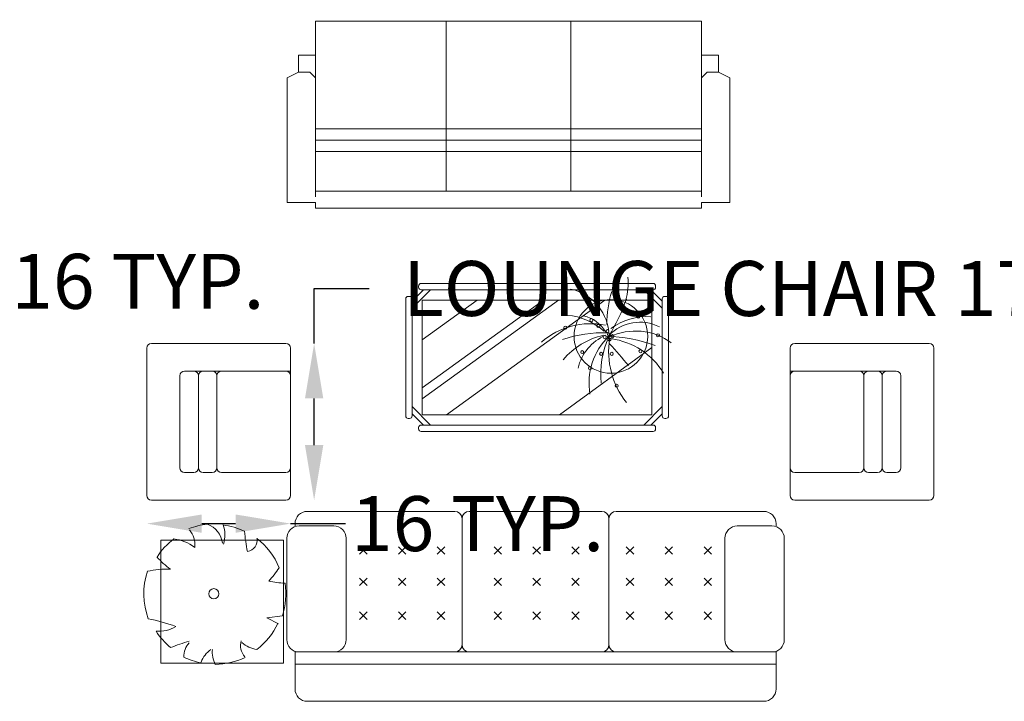
# Model space of a CAD drawing. Units: inches. Extents: x 1994 to 3075, y 3517 to 3950.
# Tile 55 of 58: x 2912 to 3019, y 3623 to 3698. Entities that reach past the tile are written whole.
import ezdxf

# ---------------------------------------------------------------- set-up
doc = ezdxf.new("R2010")
doc.units = ezdxf.units.IN
doc.layers.add('A-ANNO-DIMS', color=2, linetype='Continuous', lineweight=18)
doc.layers.add('A-FURN', color=8, linetype='Continuous', lineweight=18)
doc.styles.get("Standard").update_dxf_attribs({"font": 'arial.ttf'})
doc.dimstyles.get("Standard").update_dxf_attribs({"dimtxt": 6, "dimasz": 6, "dimexe": 0.18, "dimexo": 0.0625, "dimgap": 0.09, "dimtad": 0, "dimtih": 1, "dimtoh": 1, "dimdec": 4, "dimzin": 0, "dimdsep": 46, "dimlunit": 4, "dimtxsty": 'Standard', "dimcen": 0.09, "dimse1": 1, "dimse2": 1, "dimadec": 0, "dimazin": 0, "dimtfac": 1, "dimtdec": 4, "dimtofl": 0, "dimtmove": 0, "dimatfit": 3, "dimfxl": 1, "dimtolj": 1, "dimtzin": 0, "dimarcsym": 0})

# ---------------------------------------------------------------- blocks, each defined once
blk = doc.blocks.new('CHAIR-LOUNGE')
for p, q in [((0, 16.6), (0, 0.5)), ((0.5, 17.1), (15.19, 17.1)), ((15.7, 16.6), (15.7, 0.5)), ((4.12, 14.09), (15.7, 14.09)), ((3.62, 13.58), (3.62, 3.52)), ((5.63, 13.58), (5.63, 3.52)), ((7.65, 3.52), (7.65, 13.58)), ((4.12, 3.02), (5.13, 3.02)), ((6.14, 3.02), (7.14, 3.02)), ((8.15, 3.02), (15.19, 3.02)), ((0.5, 0), (15.19, 0))]:
    blk.add_line(p, q)
for centre, start, end in [((0.5, 16.6), 90, 180), ((15.19, 16.6), 0, 90), ((4.12, 13.58), 90, 180), ((5.13, 13.58), 0, 90), ((6.14, 13.58), 90, 180), ((7.14, 13.58), 0, 90), ((8.15, 13.58), 90, 180), ((15.19, 13.58), 0, 90), ((4.12, 3.52), 180, 270), ((5.13, 3.52), 270, 0), ((6.14, 3.52), 180, 270), ((7.14, 3.52), 270, 0), ((8.15, 3.52), 180, 270), ((15.19, 3.52), 270, 0), ((0.5, 0.5), 180, 270), ((15.19, 0.5), 270, 0)]:
    blk.add_arc(centre, 0.503, start, end)
blk = doc.blocks.new('*D15')
at = {"layer": 'A-ANNO-DIMS', "color": 0, "lineweight": -2, "transparency": 16777216}
for p, q in [((2835.85, 3669.06), (2840.19, 3669.06)), ((2846.19, 3669.06), (2852.19, 3669.06))]:
    blk.add_line(p, q, dxfattribs=at)
at = {"layer": 'A-ANNO-DIMS', "color": 0, "transparency": 16777216}
for points in [[(2835.85, 3670.06), (2835.85, 3668.06), (2829.85, 3669.06)], [(2840.19, 3670.06), (2840.19, 3668.06), (2846.19, 3669.06)]]:
    blk.add_solid(points, dxfattribs=at)
at = {"layer": 'Defpoints', "color": 0, "transparency": 16777216}
for p in [(2829.85, 3671.51), (2846.19, 3671.51), (2846.19, 3669.06)]:
    blk.add_point(p, dxfattribs=at)
at = {"layer": 'A-ANNO-DIMS', "color": 0, "transparency": 16777216, "insert": (2896.77, 3669.06), "char_height": 6, "attachment_point": 5}
blk.add_mtext('\\A1;DINING CHAIR 16 TYP.', dxfattribs=at)
blk = doc.blocks.new('*D25')
at = {"layer": 'A-ANNO-DIMS', "color": 0, "lineweight": -2, "transparency": 16777216}
for p, q in [((2943.67, 3662.28), (2943.67, 3668.28)), ((2943.67, 3668.28), (2949.67, 3668.28)), ((2943.67, 3651.18), (2943.67, 3656.28))]:
    blk.add_line(p, q, dxfattribs=at)
at = {"layer": 'A-ANNO-DIMS', "color": 0, "transparency": 16777216}
for points in [[(2942.67, 3656.28), (2944.67, 3656.28), (2943.67, 3662.28)], [(2942.67, 3651.18), (2944.67, 3651.18), (2943.67, 3645.18)]]:
    blk.add_solid(points, dxfattribs=at)
at = {"layer": 'Defpoints', "color": 0, "transparency": 16777216}
for p in [(2941.1, 3662.28), (2943.67, 3662.28), (2941.1, 3645.18)]:
    blk.add_point(p, dxfattribs=at)
at = {"layer": 'A-ANNO-DIMS', "color": 0, "transparency": 16777216, "insert": (2997.3, 3668.28), "char_height": 6, "attachment_point": 5}
blk.add_mtext('\\A1;LOUNGE CHAIR 17 TYP.', dxfattribs=at)
blk = doc.blocks.new('*D26')
at = {"layer": 'A-ANNO-DIMS', "color": 0, "lineweight": -2, "transparency": 16777216}
for p, q in [((2931.41, 3642.61), (2935.1, 3642.61)), ((2941.1, 3642.61), (2947.1, 3642.61))]:
    blk.add_line(p, q, dxfattribs=at)
at = {"layer": 'A-ANNO-DIMS', "color": 0, "transparency": 16777216}
for points in [[(2931.41, 3643.61), (2931.41, 3641.61), (2925.41, 3642.61)], [(2935.1, 3643.61), (2935.1, 3641.61), (2941.1, 3642.61)]]:
    blk.add_solid(points, dxfattribs=at)
at = {"layer": 'Defpoints', "color": 0, "transparency": 16777216}
for p in [(2925.41, 3645.18), (2941.1, 3645.18), (2941.1, 3642.61)]:
    blk.add_point(p, dxfattribs=at)
at = {"layer": 'A-ANNO-DIMS', "color": 0, "transparency": 16777216, "insert": (2961.51, 3642.61), "char_height": 6, "attachment_point": 5}
blk.add_mtext('\\A1;16 TYP.', dxfattribs=at)
blk = doc.blocks.new('*D27')
at = {"layer": 'A-ANNO-DIMS', "color": 0, "lineweight": -2, "transparency": 16777216}
for p, q in [((2981.58, 3712.96), (2981.58, 3712.87)), ((2981.58, 3706.38), (2981.58, 3706.48))]:
    blk.add_line(p, q, dxfattribs=at)
at = {"layer": 'A-ANNO-DIMS', "color": 0, "transparency": 16777216}
for points in [[(2980.58, 3712.96), (2982.58, 3712.96), (2981.58, 3718.96)], [(2980.58, 3706.38), (2982.58, 3706.38), (2981.58, 3700.38)]]:
    blk.add_solid(points, dxfattribs=at)
at = {"layer": 'Defpoints', "color": 0, "transparency": 16777216}
for p in [(2984.36, 3718.96), (2981.58, 3700.38), (2984.36, 3700.38)]:
    blk.add_point(p, dxfattribs=at)
at = {"layer": 'A-ANNO-DIMS', "color": 0, "transparency": 16777216, "insert": (2981.58, 3709.67), "char_height": 6, "attachment_point": 5}
blk.add_mtext('\\A1;SIDE CHAIR 19 TYP.', dxfattribs=at)

msp = doc.modelspace()

# ---------------------------------------------------------------- linework, layer by layer
at = {"layer": 'A-FURN'}
for p, q in [((2943.833, 3697.4715), (2943.833, 3678.2684)), ((2985.9559, 3697.4715), (2943.833, 3697.4715)), ((2958.0805, 3697.4715), (2958.0805, 3678.8879)), ((2971.7084, 3697.4715), (2971.7084, 3678.8879)), ((2985.9559, 3697.4715), (2985.9559, 3678.2684)), ((2943.833, 3693.7548), (2941.9746, 3693.7548)), ((2941.9746, 3693.7548), (2941.9746, 3691.8964)), ((2987.8143, 3693.7548), (2985.9559, 3693.7548)), ((2987.8143, 3691.8964), (2987.8143, 3693.7548)), ((2941.9746, 3691.8964), (2940.7357, 3691.277)), ((2941.9746, 3691.8964), (2943.2136, 3691.8964)), ((2943.2136, 3691.8964), (2943.833, 3691.277)), ((2986.5754, 3691.8964), (2985.9559, 3691.277)), ((2987.8143, 3691.8964), (2986.5754, 3691.8964)), ((2989.0532, 3691.277), (2987.8143, 3691.8964)), ((2940.7357, 3691.277), (2940.7357, 3677.649)), ((2989.0532, 3677.649), (2989.0532, 3691.277)), ((2985.9559, 3685.7019), (2943.833, 3685.7019)), ((2985.9559, 3684.463), (2943.833, 3684.463)), ((2985.9559, 3683.2241), (2943.833, 3683.2241)), ((2943.833, 3678.8879), (2985.9559, 3678.8879)), ((2940.7357, 3677.649), (2943.833, 3677.649)), ((2943.833, 3677.649), (2943.833, 3677.0295)), ((2943.833, 3677.0295), (2985.9559, 3677.0295)), ((2985.9559, 3677.0295), (2985.9559, 3677.649)), ((2985.9559, 3677.649), (2989.0532, 3677.649)), ((2956.3786, 3668.1312), (2954.3653, 3666.1179)), ((2955.5909, 3668.1312), (2954.3653, 3666.9056)), ((2955.0776, 3668.549), (2955.0776, 3668.4097)), ((2955.3561, 3668.8275), (2980.6682, 3668.8275)), ((2955.3561, 3668.1312), (2980.6682, 3668.1312)), ((2979.6457, 3668.1312), (2981.659, 3666.1179)), ((2980.4334, 3668.1312), (2981.659, 3666.9056)), ((2980.9467, 3668.549), (2980.9467, 3668.4097)), ((2953.669, 3654.3612), (2953.669, 3667.1404)), ((2953.9475, 3667.4189), (2954.0868, 3667.4189)), ((2954.3653, 3654.3612), (2954.3653, 3667.1404)), ((2981.659, 3667.1404), (2981.659, 3654.3612)), ((2982.0768, 3667.4189), (2981.9375, 3667.4189)), ((2982.3553, 3667.1404), (2982.3553, 3654.3612)), ((2955.4793, 3656.2225), (2970.3399, 3667.0172)), ((2955.4793, 3657.4188), (2968.693, 3667.0172)), ((2955.4793, 3662.6734), (2961.4592, 3667.0172)), ((2955.4793, 3654.4844), (2955.4793, 3667.0172)), ((2955.4793, 3667.0172), (2980.545, 3667.0172)), ((2958.1325, 3654.4844), (2975.3859, 3667.0172)), ((2980.545, 3667.0172), (2980.545, 3654.4844)), ((2970.4453, 3654.4844), (2980.545, 3661.8208)), ((2956.3786, 3653.3703), (2954.3653, 3655.3837)), ((2979.6457, 3653.3703), (2981.659, 3655.3837)), ((2955.5909, 3653.3703), (2954.3653, 3654.5959)), ((2980.545, 3654.4844), (2955.4793, 3654.4844)), ((2980.4334, 3653.3703), (2981.659, 3654.5959)), ((2953.9475, 3654.0827), (2954.0868, 3654.0827)), ((2955.0776, 3652.9526), (2955.0776, 3653.0918)), ((2980.6682, 3653.3703), (2955.3561, 3653.3703)), ((2980.9467, 3652.9526), (2980.9467, 3653.0918)), ((2982.0768, 3654.0827), (2981.9375, 3654.0827)), ((2980.6682, 3652.6741), (2955.3561, 3652.6741)), ((2942.932, 3643.9457), (2959.0378, 3643.9457)), ((2960.6024, 3643.9457), (2975.074, 3643.9457)), ((2976.6386, 3643.9457), (2992.7443, 3643.9457)), ((2941.5858, 3642.3608), (2941.5858, 3642.5995)), ((2942.0319, 3642.3608), (2945.8188, 3642.3608)), ((2959.8201, 3643.1384), (2959.8201, 3629.406)), ((2975.8563, 3643.1384), (2975.8563, 3629.406)), ((2993.6444, 3642.3608), (2989.8575, 3642.3608)), ((2994.0906, 3642.3608), (2994.0906, 3642.5995)), ((2926.9262, 3627.3737), (2926.9262, 3640.7908)), ((2926.9262, 3640.7908), (2940.3433, 3640.7908)), ((2940.3433, 3640.7908), (2940.3433, 3627.3737)), ((2940.6856, 3629.9445), (2940.6856, 3641.0145)), ((2947.1651, 3641.0145), (2947.1651, 3629.9445)), ((2988.5113, 3641.0145), (2988.5113, 3629.9445)), ((2994.9907, 3629.9445), (2994.9907, 3641.0145)), ((2949.4419, 3640.0866), (2948.6296, 3639.2743)), ((2948.6296, 3640.0866), (2949.4419, 3639.2743)), ((2953.6852, 3640.0866), (2952.8729, 3639.2743)), ((2952.8729, 3640.0866), (2953.6852, 3639.2743)), ((2957.9285, 3640.0866), (2957.1162, 3639.2743)), ((2957.1162, 3640.0866), (2957.9285, 3639.2743)), ((2963.309, 3640.0866), (2964.1213, 3639.2743)), ((2964.1213, 3640.0866), (2963.309, 3639.2743)), ((2967.5523, 3640.0866), (2968.3646, 3639.2743)), ((2968.3646, 3640.0866), (2967.5523, 3639.2743)), ((2971.7956, 3640.0866), (2972.6079, 3639.2743)), ((2972.6079, 3640.0866), (2971.7956, 3639.2743)), ((2978.5602, 3640.0866), (2977.7479, 3639.2743)), ((2977.7479, 3640.0866), (2978.5602, 3639.2743)), ((2982.8035, 3640.0866), (2981.9912, 3639.2743)), ((2981.9912, 3640.0866), (2982.8035, 3639.2743)), ((2987.0467, 3640.0866), (2986.2344, 3639.2743)), ((2986.2344, 3640.0866), (2987.0467, 3639.2743)), ((2949.4419, 3636.6669), (2948.6296, 3635.8546)), ((2948.6296, 3636.6669), (2949.4419, 3635.8546)), ((2953.6852, 3636.6669), (2952.8729, 3635.8546)), ((2952.8729, 3636.6669), (2953.6852, 3635.8546)), ((2957.9285, 3636.6669), (2957.1162, 3635.8546)), ((2957.1162, 3636.6669), (2957.9285, 3635.8546)), ((2963.309, 3636.6669), (2964.1213, 3635.8546)), ((2964.1213, 3636.6669), (2963.309, 3635.8546)), ((2967.5523, 3636.6669), (2968.3646, 3635.8546)), ((2968.3646, 3636.6669), (2967.5523, 3635.8546)), ((2971.7956, 3636.6669), (2972.6079, 3635.8546)), ((2972.6079, 3636.6669), (2971.7956, 3635.8546)), ((2978.5602, 3636.6669), (2977.7479, 3635.8546)), ((2977.7479, 3636.6669), (2978.5602, 3635.8546)), ((2982.8035, 3636.6669), (2981.9912, 3635.8546)), ((2981.9912, 3636.6669), (2982.8035, 3635.8546)), ((2987.0467, 3636.6669), (2986.2344, 3635.8546)), ((2986.2344, 3636.6669), (2987.0467, 3635.8546)), ((2949.4419, 3632.9736), (2948.6296, 3632.1613)), ((2948.6296, 3632.9736), (2949.4419, 3632.1613)), ((2952.8729, 3632.9736), (2953.6852, 3632.1613)), ((2953.6852, 3632.9736), (2952.8729, 3632.1613)), ((2957.9285, 3632.9736), (2957.1162, 3632.1613)), ((2957.1162, 3632.9736), (2957.9285, 3632.1613)), ((2963.309, 3632.9736), (2964.1213, 3632.1613)), ((2964.1213, 3632.9736), (2963.309, 3632.1613)), ((2968.3646, 3632.9736), (2967.5523, 3632.1613)), ((2967.5523, 3632.9736), (2968.3646, 3632.1613)), ((2971.7956, 3632.9736), (2972.6079, 3632.1613)), ((2972.6079, 3632.9736), (2971.7956, 3632.1613)), ((2978.5602, 3632.9736), (2977.7479, 3632.1613)), ((2977.7479, 3632.9736), (2978.5602, 3632.1613)), ((2981.9912, 3632.9736), (2982.8035, 3632.1613)), ((2982.8035, 3632.9736), (2981.9912, 3632.1613)), ((2987.0467, 3632.9736), (2986.2344, 3632.1613)), ((2986.2344, 3632.9736), (2987.0467, 3632.1613)), ((2940.2002, 3632.5581), (2938.4968, 3632.3296)), ((2938.4968, 3632.3296), (2939.7691, 3631.6814)), ((2941.5858, 3624.5594), (2941.5858, 3628.6743)), ((2994.0906, 3628.5982), (2941.5858, 3628.5982)), ((2994.0906, 3628.5982), (2994.0906, 3624.5594)), ((2940.3433, 3627.3737), (2926.9262, 3627.3737)), ((2994.0906, 3627.2519), (2941.5858, 3627.2519)), ((2992.7443, 3623.2131), (2942.932, 3623.2131))]:
    msp.add_line(p, q, dxfattribs=at)
for centre, radius in [((2976.0594, 3663.0507), 4.0196), ((2973.9283, 3664.8216), 0.1671), ((2979.0586, 3665.1899), 0.1671), ((2971.0956, 3663.9954), 0.1671), ((2974.6942, 3664.1795), 0.1671), ((2975.3826, 3662.985), 0.1671), ((2975.6895, 3663.6271), 0.1671), ((2975.843, 3663.2604), 0.1671), ((2975.919, 3662.7096), 0.1671), ((2976.2246, 3663.0763), 0.1671), ((2981.2014, 3663.1692), 0.1671), ((2972.9329, 3661.331), 0.1671), ((2974.9997, 3661.1469), 0.1671), ((2976.1485, 3661.1469), 0.1671), ((2979.2881, 3661.4223), 0.1671), ((2973.7748, 3659.5857), 0.1671), ((2976.6849, 3657.6563), 0.1671), ((2932.7283, 3634.9579), 0.5534)]:
    msp.add_circle(centre, radius, dxfattribs=at)
for centre, radius, start, end in [((2971.8422, 3668.819), 6.1066, 342.945635, 6.481378), ((2955.3561, 3668.549), 0.2785, 90, 180), ((2955.3561, 3668.4097), 0.2785, 180, 270), ((2970.5178, 3662.9741), 5.3651, 6.990448, 78.028363), ((2980.6682, 3668.549), 0.2785, 0, 90), ((2980.6682, 3668.4097), 0.2785, 270, 0), ((2953.9475, 3667.1404), 0.2785, 90, 180), ((2954.0868, 3667.1404), 0.2785, 0, 90), ((2989.2543, 3664.1518), 13.6438, 163.856122, 179.110515), ((2956.4997, 3674.7047), 22.5695, 328.987278, 340.361011), ((2981.9375, 3667.1404), 0.2785, 90, 180), ((2982.0768, 3667.1404), 0.2785, 0, 90), ((2970.5544, 3658.2067), 7.2086, 48.758099, 83.862401), ((2972.3832, 3661.838), 3.5142, 28.890119, 78.457922), ((2979.9704, 3658.7231), 6.4836, 85.874061, 126.95584), ((2973.8412, 3656.2772), 8.1559, 78.551551, 130.981535), ((2979.2198, 3659.898), 4.7015, 62.990858, 135.910172), ((2975.2814, 3649.4586), 13.9919, 88.328565, 108.729003), ((2977.0604, 3655.2659), 8.1127, 103.045235, 139.776625), ((2977.6244, 3658.3297), 5.3014, 114.095577, 166.295338), ((2980.9118, 3657.9156), 7.2337, 134.486062, 189.376218), ((2984.571, 3658.9315), 9.6234, 155.08876, 185.963724), ((2974.9332, 3645.2045), 17.8846, 70.524897, 87.824368), ((2984.8705, 3661.4231), 9.0569, 171.249582, 218.23328), ((2978.7571, 3657.1046), 6.5295, 53.32313, 115.763258), ((2974.9779, 3654.8745), 8.0016, 31.315049, 82.137794), ((2939.2692, 3628.4544), 49.8533, 39.04877, 42.6799), ((2953.9475, 3654.3612), 0.2785, 180, 270), ((2954.0868, 3654.3612), 0.2785, 270, 0), ((2981.9375, 3654.3612), 0.2785, 180, 270), ((2982.0768, 3654.3612), 0.2785, 270, 0), ((2955.3561, 3653.0918), 0.2785, 90, 180), ((2980.6682, 3653.0918), 0.2785, 0, 90), ((2955.3561, 3652.9526), 0.2785, 180, 270), ((2980.6682, 3652.9526), 0.2785, 270, 0), ((2942.932, 3642.5995), 1.3463, 90, 180), ((2959.0123, 3643.1384), 0.8078, 0, 90), ((2960.6278, 3643.1384), 0.8078, 90, 180), ((2975.0485, 3643.1384), 0.8078, 0, 90), ((2976.664, 3643.1384), 0.8078, 90, 180), ((2992.7443, 3642.5995), 1.3463, 0, 90), ((2932.8043, 3634.9551), 7.6406, 95.923625, 111.527702), ((2931.1212, 3640.1371), 2.578, 7.391154, 69.695169), ((2932.8043, 3634.9551), 7.5625, 64.349833, 83.035621), ((2930.7372, 3641.3713), 3.1922, 341.800851, 20.599149), ((2942.0319, 3641.0145), 1.3463, 90, 180), ((2945.8188, 3641.0145), 1.3463, 0, 90), ((2989.8575, 3641.0145), 1.3463, 90, 180), ((2993.6444, 3641.0145), 1.3463, 0, 90), ((2928.286, 3640.3558), 2.3685, 351.831375, 41.827816), ((2952.089, 3642.9331), 16.053, 184.146464, 192.123814), ((2932.8043, 3634.9551), 7.4492, 126.594039, 147.446376), ((2927.9323, 3636.608), 4.3493, 51.658233, 84.30928), ((2936.1976, 3640.81), 1.2638, 278.94104, 10.010745), ((2932.8043, 3634.9551), 7.5966, 22.010297, 52.639163), ((2932.4927, 3644.1371), 7.9007, 220.853588, 235.192991), ((2932.8043, 3634.9551), 7.7319, 161.530732, 200.629966), ((2927.6423, 3628.1563), 9.4998, 87.945495, 103.214626), ((2932.5958, 3642.2403), 8.5018, 315.978173, 328.531467), ((2941.236, 3648.8328), 12.7534, 258.572822, 266.664893), ((2932.8043, 3634.9551), 7.7746, 342.042609, 8.475005), ((2919.4257, 3604.4203), 28.4809, 71.286489, 77.545106), ((2932.8043, 3634.9551), 7.6324, 307.275083, 334.82454), ((2926.7274, 3634.2385), 3.3843, 264.732262, 302.854398), ((2932.8043, 3634.9551), 7.583, 212.609838, 230.67525), ((2936.8081, 3607.1269), 23.6509, 106.639749, 111.909938), ((2931.6696, 3628.0771), 2.227, 137.045394, 180.965052), ((2937.5176, 3629.3175), 1.8838, 164.855493, 220.959999), ((2937.8954, 3632.0995), 3.2517, 229.720325, 261.715134), ((2942.0319, 3629.9445), 1.3463, 180, 270), ((2945.8188, 3629.9445), 1.3463, 270, 0), ((2989.8575, 3629.9445), 1.3463, 180, 270), ((2993.6444, 3629.9445), 1.3463, 270, 0), ((2934.086, 3626.4882), 2.9248, 125.386829, 159.741103), ((2935.35, 3628.549), 2.7972, 173.277489, 207.812844), ((2959.0123, 3629.406), 0.8078, 270, 0), ((2960.6278, 3629.406), 0.8078, 180, 270), ((2975.0485, 3629.406), 0.8078, 270, 0), ((2976.664, 3629.406), 0.8078, 180, 270), ((2932.8043, 3634.9551), 7.6892, 244.076655, 258.902132), ((2932.8043, 3634.9551), 7.7116, 270.532148, 295.585638), ((2942.932, 3624.5594), 1.3463, 180, 270), ((2992.7443, 3624.5594), 1.3463, 270, 0)]:
    msp.add_arc(centre, radius, start, end, dxfattribs=at)

# ---------------------------------------------------------------- block references
msp.add_blockref('CHAIR-LOUNGE', (2925.408, 3645.177), dxfattribs=at)
at = {"layer": 'A-FURN', "extrusion": (0, 0, -1), "zscale": -1}
msp.add_blockref('CHAIR-LOUNGE', (-3011.3212, 3645.177), dxfattribs=at)

# ---------------------------------------------------------------- dimensions: what is measured, and where the dimension line sits
at = {"layer": 'A-ANNO-DIMS'}
for base, p1, p2, angle, text, picture, middle in [((2981.5753, 3700.381), (2984.3628, 3718.9646), (2984.3628, 3700.381), 270, 'SIDE CHAIR <> TYP.', '*D27', (2981.5753, 3709.6728)), ((2846.1884, 3669.062), (2829.8543, 3671.5122), (2846.1884, 3671.5122), 360, 'DINING CHAIR <> TYP.', '*D15', (2896.7689, 3669.062)), ((2943.6687, 3662.2807), (2941.1031, 3645.1769), (2941.1031, 3662.2807), 90, 'LOUNGE CHAIR <> TYP.', '*D25', (2997.2962, 3668.2807))]:
    dim = msp.add_linear_dim(base=base, p1=p1, p2=p2, angle=angle, text=text, dimstyle='Standard', override={"dimdec": 0, "dimlfac": 1, "dimrnd": 0, "dimzin": 0, "dimdsep": 46, "dimlunit": 2}, dxfattribs=at)
    dim.commit()
    dim.dimension.update_dxf_attribs({"geometry": picture, "text_midpoint": middle})
dim = msp.add_linear_dim(base=(2941.1031, 3642.6113), p1=(2925.4078, 3645.1769), p2=(2941.1031, 3645.1769), text='<> TYP.', dimstyle='Standard', override={"dimdec": 0, "dimlfac": 1, "dimrnd": 0, "dimzin": 0, "dimdsep": 46, "dimlunit": 2}, dxfattribs=at)
dim.commit()
dim.dimension.update_dxf_attribs({"geometry": '*D26', "text_midpoint": (2961.5137, 3642.6113)})

doc.saveas('drawing.dxf')
